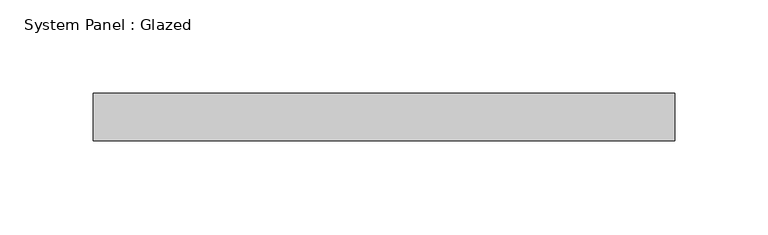
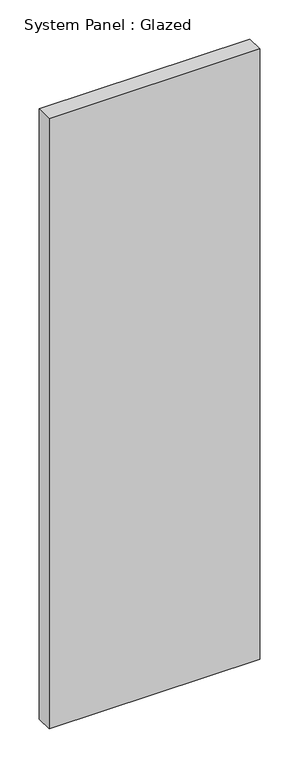
"""IFC4 building model written with IfcOpenShell, lengths in millimetres: plate geometry, System Panel : Glazed."""

from ifc_helpers import new_model, si_unit, origin, origin_with_axes, place, context, project, spatial, polyline, outline, extrude, source, transform, mapped, element, save


def system_panel_glazed_0360dae9(model_context):
    return source(origin(), model_context, "Body", "SweptSolid", [
        extrude(outline(polyline([(155.575, 19.05), (-155.575, 19.05), (-155.575, 44.45), (155.575, 44.45), (155.575, 19.05)])), origin_with_axes(), (0.0, 0.0, 1.0), 952.5),
    ])


if __name__ == "__main__":
    model = new_model("IFC4")
    model_context = context("Model", 3, world=origin())
    ifc_project = project(units=[si_unit("LENGTHUNIT", "METRE", prefix="MILLI")], contexts=[model_context])
    site = spatial("IfcSite", under=ifc_project)
    building = spatial("IfcBuilding", under=site)
    placement = place(None, origin())
    system_panel_glazed_shape = system_panel_glazed_0360dae9(model_context)
    element("IfcPlate", 1, ObjectType="System Panel : Glazed", at=placement, inside=building, context=model_context, shape_type="MappedRepresentation", body=[
        mapped(system_panel_glazed_shape, transform((0.0, 0.0, 0.0), x_axis=(1.0, 0.0, 0.0), y_axis=(0.0, 1.0, 0.0), z_axis=(0.0, 0.0, 1.0))),
    ])
    save(model, "model.ifc")

# Revit data of these elements
# Type "System Panel : Glazed"
#   Construction Type Id = "GSP4R"
#   Analytic Construction = "1/8 in Pilkington single glazing"
#   Visual Light Transmittance = 0.9
#   Solar Heat Gain Coefficient = 0.86
#   Heat Transfer Coefficient (U) = 1.18115 BTU/(h·ft²·°F)
#   Define Thermal Properties by = 1
# Element 1 (IfcPlate, "System Panel : Glazed")
#   Materials on its faces: "Glass"
# Materials
#   "Glass": class "Glass", colour RGB 0 128 192, transparency 0.75, Description = "Soda Lime Glass", Cost = 0
